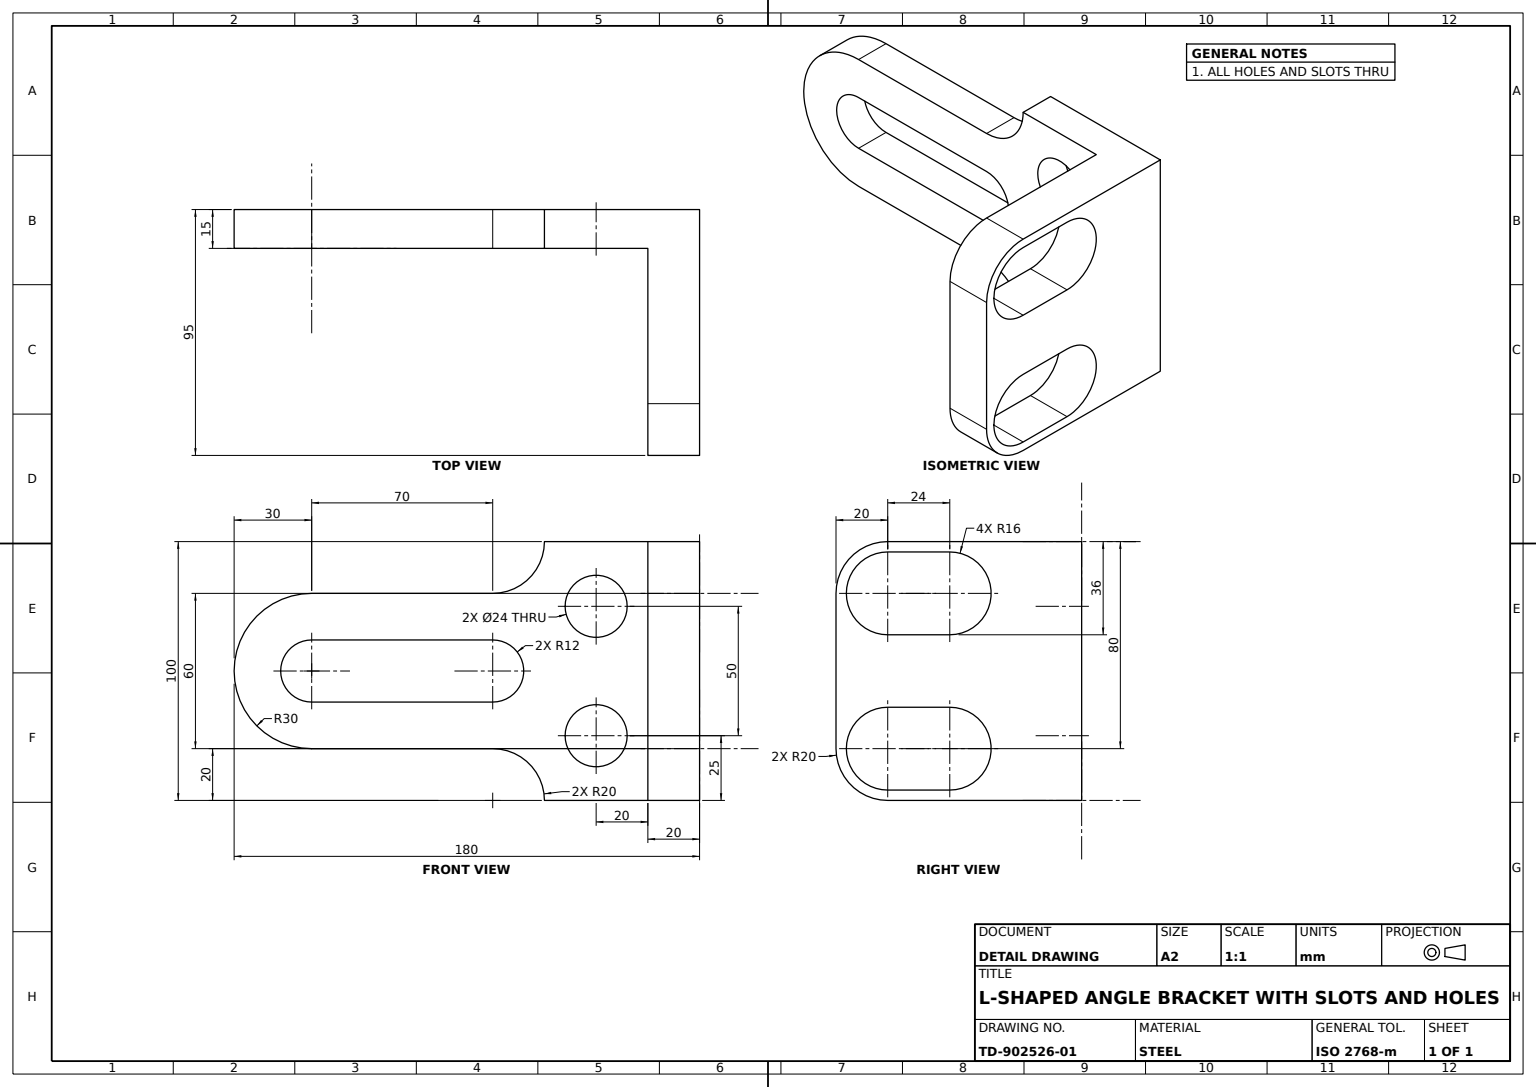
from build123d import *

# Parameters (mm, degrees)
BASE_BLOCK_DEPTH    = 20
UPRIGHT_PLATE_DEPTH = 15
SLOTTED_ARM_DEPTH   = 15
HOLES_2X_SKETCH_R   = 12
HOLES_2X_DEPTH      = 15
SLOTS_2X_DEPTH      = 20


with BuildPart() as part:
    # Base Block Sketch → Base Block (new body)
    with BuildSketch(Plane.XY):
        with BuildLine():
            Line((0, 0), (60, 0))
            ThreePointArc((60, 0), (74.142135624, 5.857864376), (80, 20))
            Line((80, 20), (80, 80))
            ThreePointArc((80, 80), (74.142135624, 94.142135624), (60, 100))
            Line((60, 100), (0, 100))
            Line((0, 100), (0, 0))
        make_face()
    extrude(amount=BASE_BLOCK_DEPTH)

    # Upright Plate Sketch → Upright Plate (add)
    with BuildSketch(Plane.ZY):
        Polygon((20, 0), (60, 0), (60, 100), (0, 100), (0, 0), align=None)
    extrude(amount=UPRIGHT_PLATE_DEPTH)

    # Slotted Arm Sketch → Slotted Arm (add)
    with BuildSketch(Plane.ZY.offset(15)):
        with BuildLine():
            Line((150, 80), (80, 80))
            ThreePointArc((80, 80), (65.857864376, 85.857864376), (60, 100))
            Line((60, 100), (60, 0))
            ThreePointArc((60, 0), (65.857864376, 14.142135624), (80, 20))
            Line((80, 20), (150, 20))
            ThreePointArc((150, 20), (180, 50), (150, 80))
        make_face()
        with BuildLine():
            Line((80, 62), (150, 62))
            ThreePointArc((150, 62), (162, 50), (150, 38))
            Line((150, 38), (80, 38))
            ThreePointArc((80, 38), (68, 50), (80, 62))
        make_face(mode=Mode.SUBTRACT)
    extrude(amount=-SLOTTED_ARM_DEPTH)

    # Holes 2x Sketch → Holes 2x (cut)
    with BuildSketch(Plane(origin=(0, 0, 0), x_dir=(0, 0, -1), z_dir=(1, 0, 0))):
        with Locations((-40, 75)):
            Circle(HOLES_2X_SKETCH_R)
        with Locations((-40, 25)):
            Circle(HOLES_2X_SKETCH_R)
    extrude(amount=-HOLES_2X_DEPTH, mode=Mode.SUBTRACT)

    # Slots 2x Sketch → Slots 2x (cut)
    with BuildSketch(Plane.XY.offset(20)):
        with BuildLine():
            Line((36, 96), (60, 96))
            ThreePointArc((60, 96), (76, 80), (60, 64))
            Line((60, 64), (36, 64))
            ThreePointArc((36, 64), (20, 80), (36, 96))
        make_face()
        with BuildLine():
            Line((36, 36), (60, 36))
            ThreePointArc((60, 36), (76, 20), (60, 4))
            Line((60, 4), (36, 4))
            ThreePointArc((36, 4), (20, 20), (36, 36))
        make_face()
    extrude(amount=-SLOTS_2X_DEPTH, mode=Mode.SUBTRACT)


solid = part.part
